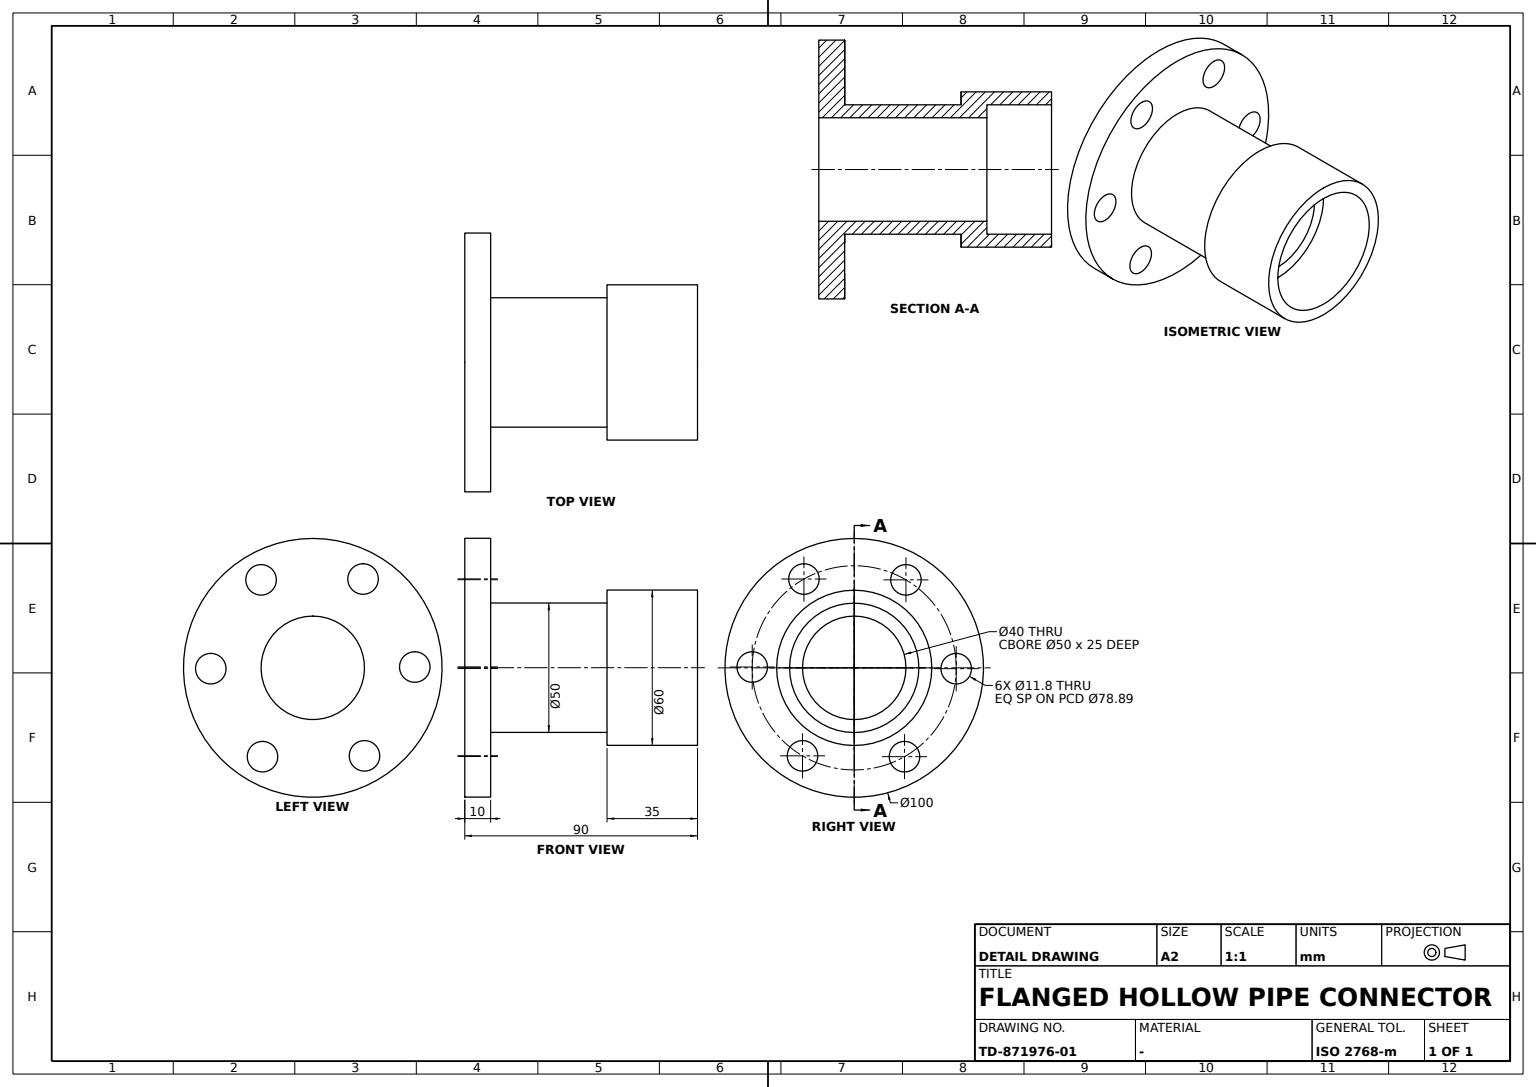
CATIA V5 part; units mm, degrees
sketch "Sketch1" plane through (0, 0, 0) normal (0, 1, 0) x (-1, 0, 0)
  point P0 (-45, 0)
  line L0 (-45, 0) -> (-45, 30)
  line L1 (-45, 30) -> (-10, 30)
  line L2 (-10, 30) -> (-10, 25)
  line L3 (-10, 25) -> (35, 25)
  line L4 (35, 25) -> (35, 50)
  line L5 (35, 50) -> (45, 50)
  line L6 (45, 50) -> (45, 0)
  line L7 (45, 0) -> (-45, 0)
  dimension "length L0" = 30
  dimension "length L1" = 35
  dimension "distance L3 L7" = 25
  dimension "distance L5 L7" = 50
  dimension "length L5" = 10
  dimension "distance L6 L0" = 90
  constraint coincidence P0 x-axis
  constraint vertical L0 y-axis
  constraint vertical L2 y-axis
  constraint vertical L4 y-axis
  constraint vertical L6 y-axis
  constraint horizontal L1 x-axis
  constraint horizontal L3 x-axis
  constraint horizontal L5 x-axis
  constraint horizontal L7 x-axis
  constraint symmetry L6 L0 y-axis
revolve "Shaft1" add sketch "Sketch1" angle 360 about L7
sketch "Sketch2" plane through (45, 0, 0) normal (1, 0, 0) x (0, 1, 0)
  circle A0 centre (0, 0) radius 25
  dimension "radius A0" = 25
extrude "Pocket1" cut sketch "Sketch2" against normal blind 25
sketch "Sketch3" plane through (20, 0, 0) normal (1, 0, 0) x (0, 1, 0)
  circle A0 centre (0, 0) radius 20
  dimension "radius A0" = 20
extrude "Pocket2" cut sketch "Sketch3" against normal blind 65
sketch "Sketch4" plane through (-35, 0, 0) normal (1, 0, 0) x (0, 1, 0)
  circle A0 centre (20, 34) radius 5.9
  point P0 (20, 34)
  dimension "radius A0" = 5.9
  dimension "distance P0 x axis" = 34
  dimension "distance P0 y axis" = 20
extrude "Pocket3" cut sketch "Sketch4" against normal blind 65
pattern_circular "CircPattern1" count 6 over 360 about axis through (0, 0, 0) along (1, 0, 0) of "Pocket3"
equation "\"angular step@CircPattern1\" = 360.0*1 deg/CircPattern1.AngularNumber"
